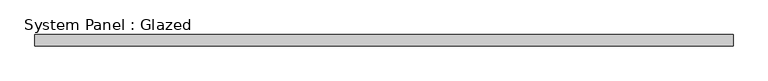
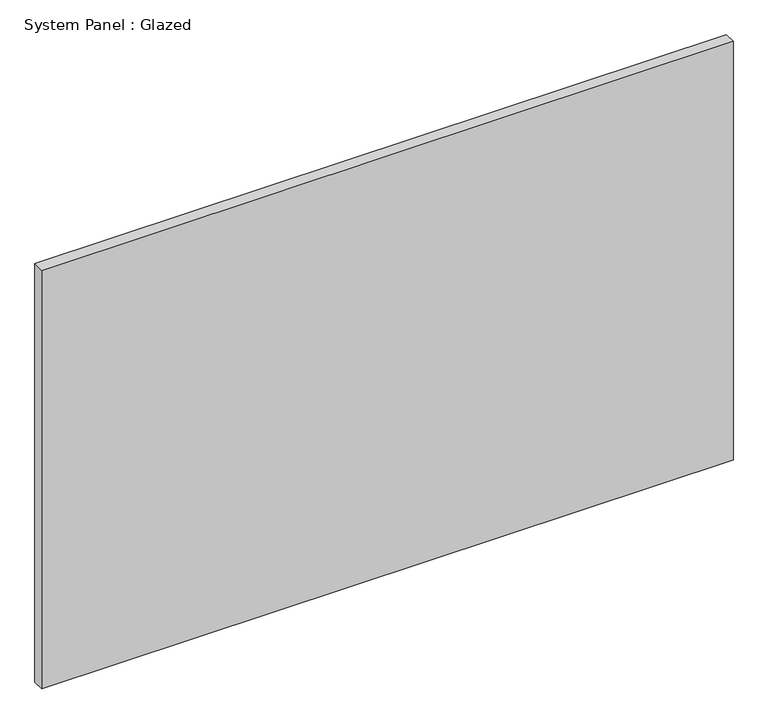
"""IFC4 building model written with IfcOpenShell, lengths in millimetres: plate geometry, System Panel : Glazed."""

from ifc_helpers import new_model, si_unit, origin, origin_with_axes, place, context, project, spatial, polyline, outline, extrude, source, transform, mapped, element, save


def system_panel_glazed_b7516aa2(model_context):
    return source(origin(), model_context, "Body", "SweptSolid", [
        extrude(outline(polyline([(765.0396696, 19.05), (-765.0396696, 19.05), (-765.0396696, 44.45), (765.0396696, 44.45), (765.0396696, 19.05)])), origin_with_axes(), (0.0, 0.0, 1.0), 979.2807647),
    ])


if __name__ == "__main__":
    model = new_model("IFC4")
    model_context = context("Model", 3, world=origin())
    ifc_project = project(units=[si_unit("LENGTHUNIT", "METRE", prefix="MILLI")], contexts=[model_context])
    site = spatial("IfcSite", under=ifc_project)
    building = spatial("IfcBuilding", under=site)
    placement = place(None, origin())
    system_panel_glazed_shape = system_panel_glazed_b7516aa2(model_context)
    element("IfcPlate", 1, ObjectType="System Panel : Glazed", at=placement, inside=building, context=model_context, shape_type="MappedRepresentation", body=[
        mapped(system_panel_glazed_shape, transform((0.0, 0.0, 0.0), x_axis=(1.0, 0.0, 0.0), y_axis=(0.0, 1.0, 0.0), z_axis=(0.0, 0.0, 1.0))),
    ])
    save(model, "model.ifc")

# Revit data of these elements
# Type "System Panel : Glazed"
#   Construction Type Id = "GSP4R"
#   Analytic Construction = "1/8 in Pilkington single glazing"
#   Visual Light Transmittance = 0.9
#   Solar Heat Gain Coefficient = 0.86
#   Heat Transfer Coefficient (U) = 1.18115 BTU/(h·ft²·°F)
#   Define Thermal Properties by = 1
# Element 1 (IfcPlate, "System Panel : Glazed")
#   Materials on its faces: "Glass"
# Materials
#   "Glass": class "Glass", colour RGB 0 128 192, transparency 0.75, Description = "Soda Lime Glass", Cost = 0
